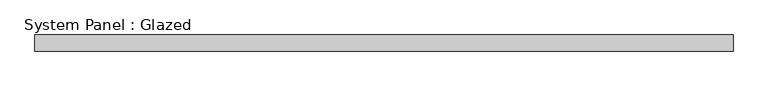
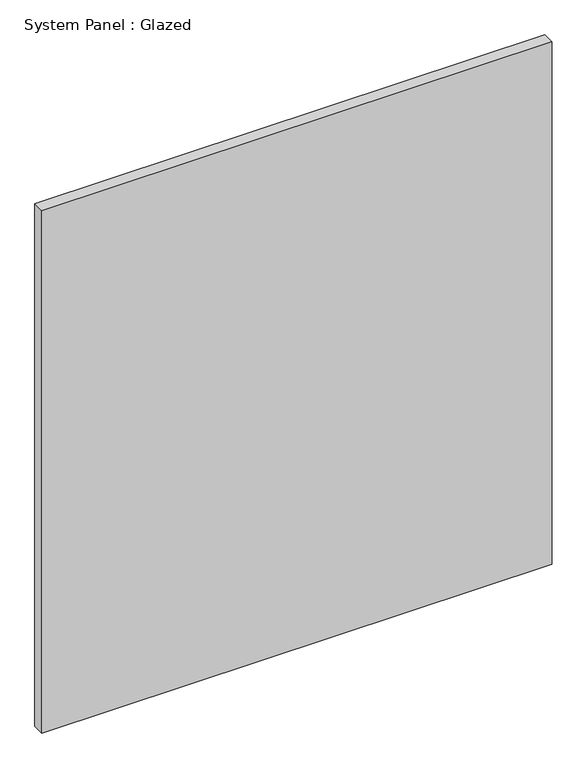
"""IFC4 building model written with IfcOpenShell, lengths in millimetres: plate geometry, System Panel : Glazed."""

from ifc_helpers import new_model, si_unit, origin, origin_with_axes, place, context, project, spatial, polyline, outline, extrude, source, transform, mapped, element, save


def system_panel_glazed_46ac4994(model_context):
    return source(origin(), model_context, "Body", "SweptSolid", [
        extrude(outline(polyline([(534.4583334, 19.05), (-534.4583334, 19.05), (-534.4583334, 44.45), (534.4583334, 44.45), (534.4583334, 19.05)])), origin_with_axes(), (0.0, 0.0, 1.0), 1155.7),
    ])


if __name__ == "__main__":
    model = new_model("IFC4")
    model_context = context("Model", 3, world=origin())
    ifc_project = project(units=[si_unit("LENGTHUNIT", "METRE", prefix="MILLI")], contexts=[model_context])
    site = spatial("IfcSite", under=ifc_project)
    building = spatial("IfcBuilding", under=site)
    placement = place(None, origin())
    system_panel_glazed_shape = system_panel_glazed_46ac4994(model_context)
    element("IfcPlate", 1, ObjectType="System Panel : Glazed", at=placement, inside=building, context=model_context, shape_type="MappedRepresentation", body=[
        mapped(system_panel_glazed_shape, transform((0.0, 0.0, 0.0), x_axis=(1.0, 0.0, 0.0), y_axis=(0.0, 1.0, 0.0), z_axis=(0.0, 0.0, 1.0))),
    ])
    save(model, "model.ifc")

# Revit data of these elements
# Type "System Panel : Glazed"
#   Construction Type Id = "GSP4R"
#   Analytic Construction = "1/8 in Pilkington single glazing"
#   Visual Light Transmittance = 0.9
#   Solar Heat Gain Coefficient = 0.86
#   Heat Transfer Coefficient (U) = 1.18115 BTU/(h·ft²·°F)
#   Define Thermal Properties by = 1
# Element 1 (IfcPlate, "System Panel : Glazed")
#   Materials on its faces: "Glass"
# Materials
#   "Glass": class "Glass", colour RGB 0 128 192, transparency 0.75, Description = "Soda Lime Glass", Cost = 0
